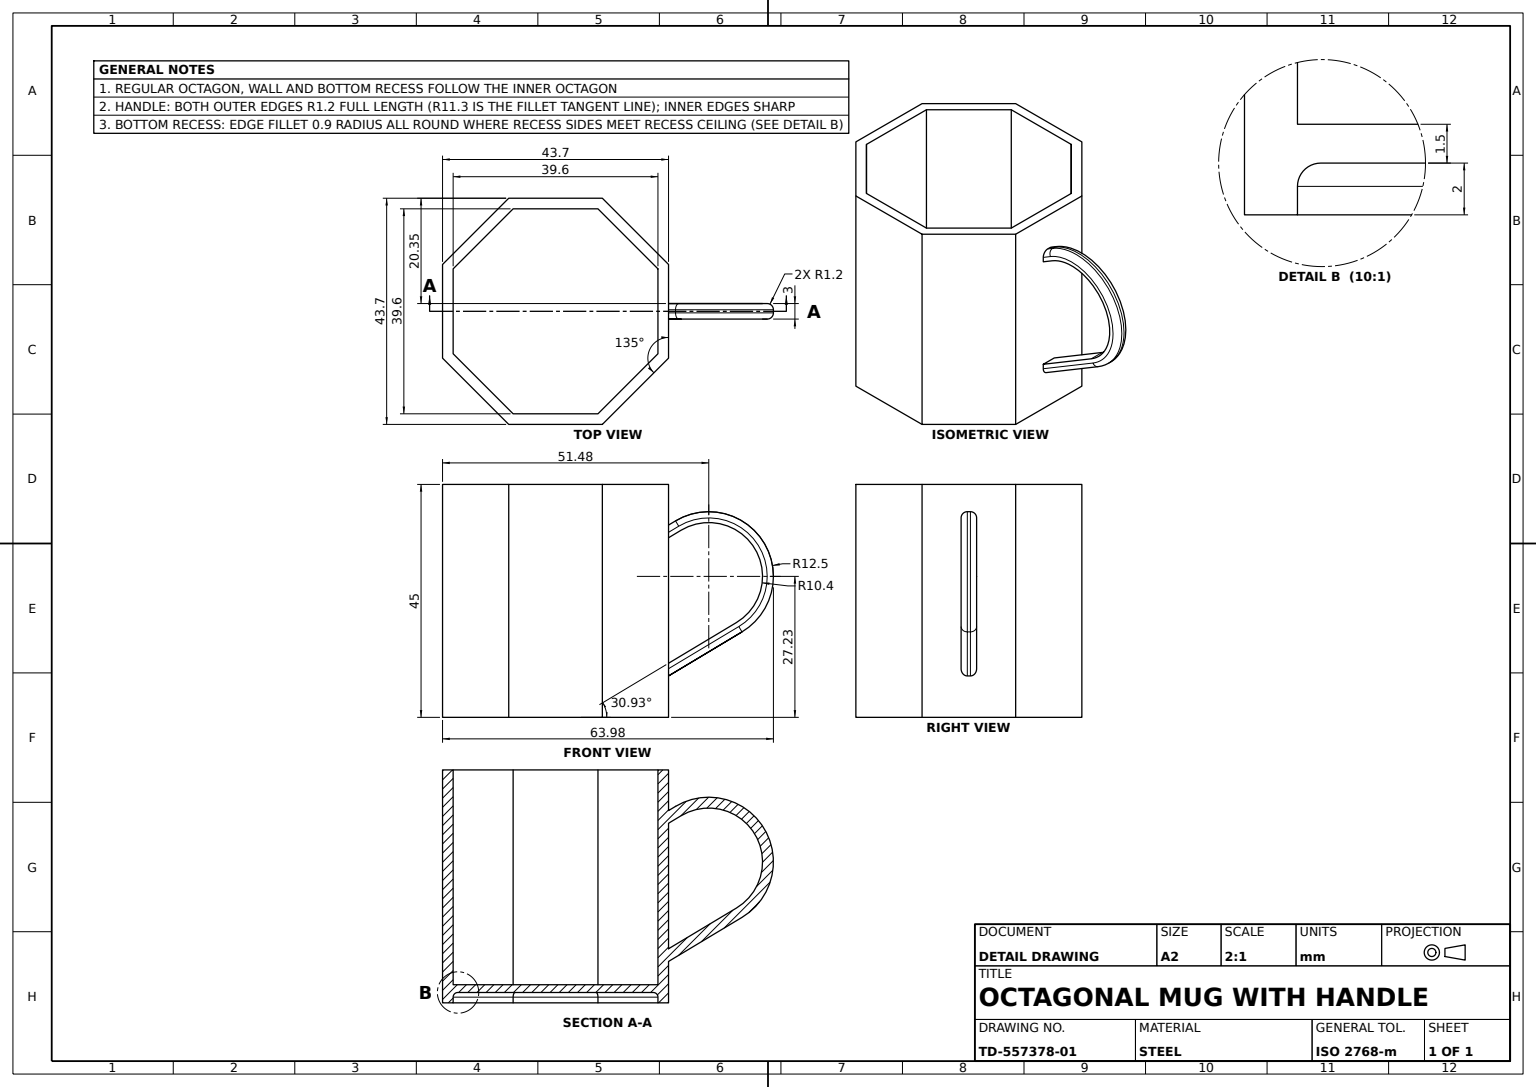
from build123d import *

# Parameters (mm, degrees)
MUG_WALL_DEPTH            = 22.5
MUG_BOTTOM_DEPTH          = 1.5
BOTTOM_EDGE_FILLET_R0_9_R = 0.9
HANDLE_DEPTH              = 1.5
HANDLE_EDGE_FILLET_R1_2_R = 1.2


with BuildPart() as part:
    # Wall Profile Octagon → Mug Wall (new, symmetric)
    with BuildSketch(Plane(origin=(0, 0, 0), x_dir=(1, 0, 0), z_dir=(0, 1, 0))):
        Polygon((21.848632739, -9.05), (21.848632739, 9.05), (9.05, 21.848632739), (-9.05, 21.848632739), (-21.848632739, 9.05), (-21.848632739, -9.05), (-9.05, -21.848632739), (9.05, -21.848632739), align=None)
        Polygon((19.8, 8.201428535), (8.201428535, 19.8), (-8.201428535, 19.8), (-19.8, 8.201428535), (-19.8, -8.201428535), (-8.201428535, -19.8), (8.201428535, -19.8), (19.8, -8.201428535), align=None, mode=Mode.SUBTRACT)
    extrude(amount=MUG_WALL_DEPTH, both=True)

    # Bottom Profile Octagon → Mug Bottom (add)
    with BuildSketch(Plane(origin=(0, -20.5, 0), x_dir=(1, 0, 0), z_dir=(0, 1, 0))):
        Polygon((-19.8, 8.201428535), (-19.8, -8.201428535), (-8.201428535, -19.8), (8.201428535, -19.8), (19.8, -8.201428535), (19.8, 8.201428535), (8.201428535, 19.8), (-8.201428535, 19.8), align=None)
    extrude(amount=MUG_BOTTOM_DEPTH)

    # Bottom Edge Fillet R0.9
    bottom_edge_fillet_r0_9_edges = [part.edges().sort_by_distance(p)[0] for p in [
        (-14.000714267, -20.5, -14.000714267),
        (-19.8, -20.5, 0),
        (-14.000714267, -20.5, 14.000714267),
        (0, -20.5, 19.8),
        (14.000714267, -20.5, 14.000714267),
        (19.8, -20.5, 0),
        (14.000714267, -20.5, -14.000714267),
        (0, -20.5, -19.8),
    ]]
    fillet(bottom_edge_fillet_r0_9_edges, radius=BOTTOM_EDGE_FILLET_R0_9_R)

    # Handle Profile → Handle (add, symmetric)
    with BuildSketch(Plane.XY):
        with BuildLine():
            Line((21.848632739, -12.051874881), (34.972961948, -4.18790751))
            ThreePointArc((34.972961948, -4.18790751), (38.548632739, 10.078647028), (24.282078201, 13.65431782))
            Line((24.282078201, 13.65431782), (21.848632739, 12.196221531))
            Line((21.848632739, 12.196221531), (21.848632739, 14.644346649))
            Line((21.848632739, 14.644346649), (23.202710131, 15.455696338))
            ThreePointArc((23.202710131, 15.455696338), (40.350011258, 11.158015099), (36.052330019, -5.989286029))
            Line((36.052330019, -5.989286029), (21.848632739, -14.5))
            Line((21.848632739, -14.5), (21.848632739, -12.051874881))
        make_face()
    extrude(amount=HANDLE_DEPTH, both=True)

    # Handle Edge Fillet R1.2
    handle_edge_fillet_r1_2_edges = [part.edges().sort_by_distance(p)[0] for p in [
        (28.950481379, -10.244643014, -1.5),
        (40.350011258, 11.158015099, -1.5),
        (22.525671435, 15.050021494, -1.5),
        (28.950481379, -10.244643014, 1.5),
        (40.350011258, 11.158015099, 1.5),
        (22.525671435, 15.050021494, 1.5),
    ]]
    fillet(handle_edge_fillet_r1_2_edges, radius=HANDLE_EDGE_FILLET_R1_2_R)


solid = part.part
